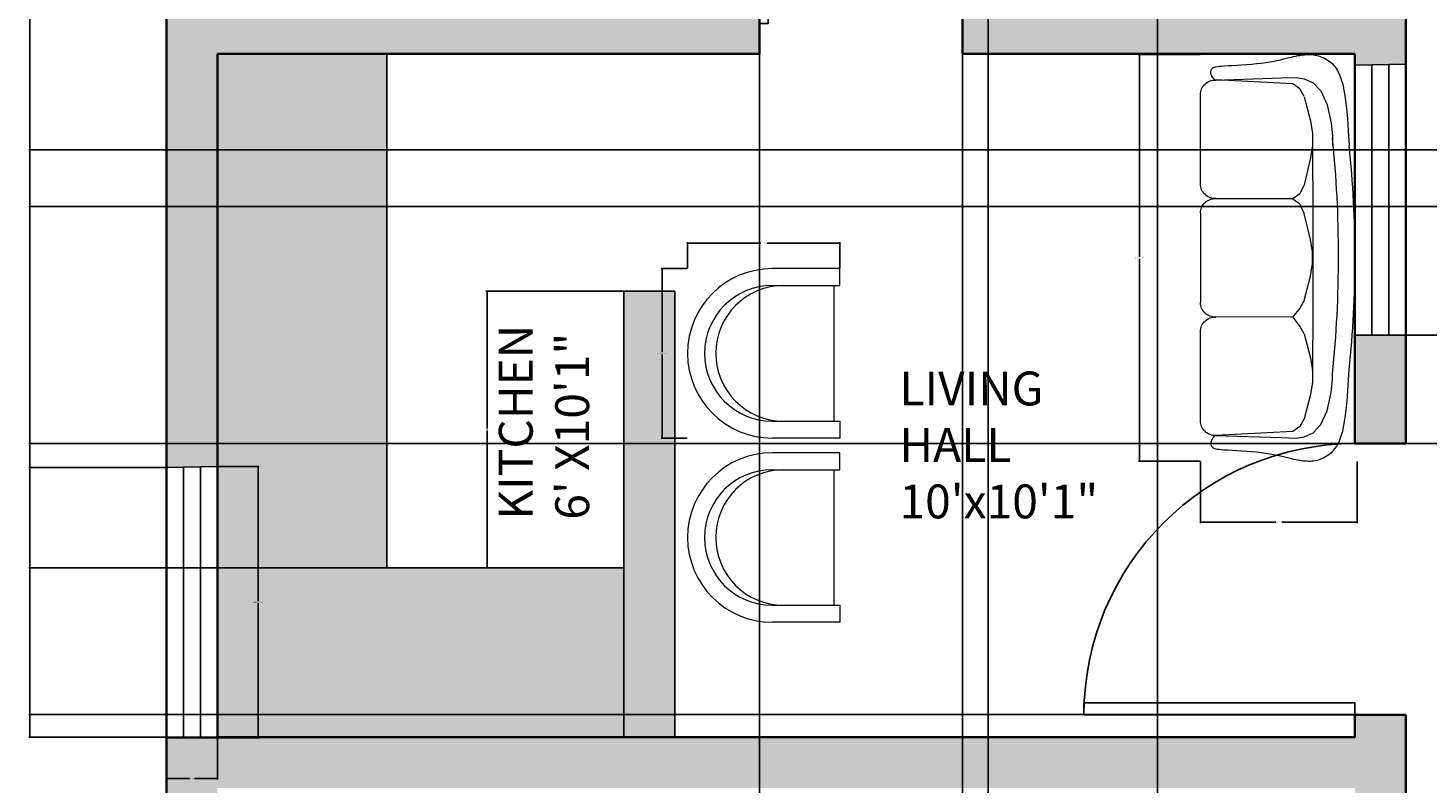
# Model space of a CAD drawing. Units: millimetres. Extents: x 2817 to 5038, y 1110 to 3565.
# Tile 10 of 21: x 2817 to 3065, y 1371 to 1505. Entities that reach past the tile are written whole.
import ezdxf

# ---------------------------------------------------------------- set-up
doc = ezdxf.new("R2010")
doc.units = ezdxf.units.MM
for name, color, linetype, lineweight in [('A-ANNO-DIMS', 2, 'Continuous', 18), ('A-AREA-IDEN', 7, 'Continuous', 18), ('A-FLOR-CASE', 7, 'Continuous', 25), ('A-WALL', 7, 'Continuous', 35), ('DOOR&WINDOW', 1, 'Continuous', 25), ('FURNITURE', 219, 'Continuous', 18)]:
    doc.layers.add(name, color=color, linetype=linetype, lineweight=lineweight)
doc.layers.add('A-FLOR-CASE-PATT', color=251, linetype='Continuous', lineweight=13, true_color=0x636466)
doc.layers.add('A-WALL-PATT', color=51, linetype='Continuous', lineweight=13, true_color=0xf7f281)
doc.styles.get("Standard").update_dxf_attribs({"font": 'arial.ttf'})
doc.dimstyles.get("Standard").update_dxf_attribs({"dimtxt": 0.18, "dimasz": 0.18, "dimexe": 0.18, "dimexo": 0.0625, "dimgap": 0.09, "dimtad": 0, "dimtih": 1, "dimtoh": 1, "dimdec": 4, "dimzin": 0, "dimdsep": 46, "dimtxsty": 'Standard', "dimcen": 0.09, "dimadec": 0, "dimazin": 0, "dimtfac": 1, "dimtdec": 4, "dimtofl": 0, "dimtmove": 0, "dimatfit": 3, "dimfxl": 1, "dimtolj": 1, "dimtzin": 0, "dimarcsym": 0})

# ---------------------------------------------------------------- blocks, each defined once
blk = doc.blocks.new('*U2')
for p, q in [((0, 0), (0, -6)), ((40, 0), (40, -6))]:
    blk.add_line(p, q)
blk.add_lwpolyline([(0, 0), (0, 40), (1.75, 40), (1.75, 0)], close=True)
blk.add_arc((0, 0), 40, 0, 90)
blk = doc.blocks.new('*U3')
for p, q in [((-40, 0), (-40, 6)), ((0, 0), (0, 6))]:
    blk.add_line(p, q)
blk.add_lwpolyline([(0, 0), (0, -40), (-1.75, -40), (-1.75, 0)], close=True)
blk.add_arc((0, 0), 40, 180, 270)
blk = doc.blocks.new('A$C2E47758B')
for p, q in [((168.6, 1918.7), (160.6, 1917.4)), ((176.5, 1919.5), (168.6, 1918.7)), ((184.4, 1919.9), (176.5, 1919.5)), ((192.3, 1919.9), (184.4, 1919.9)), ((200.2, 1919.6), (192.3, 1919.9)), ((208.2, 1919.1), (200.2, 1919.6)), ((216.4, 1918.3), (208.2, 1919.1)), ((224.7, 1917.3), (216.4, 1918.3)), ((61.4, 1854.6), (55.6, 1845.5)), ((67.4, 1862.7), (61.4, 1854.6)), ((73.8, 1870), (67.4, 1862.7)), ((80.6, 1876.8), (73.8, 1870)), ((87.8, 1883), (80.6, 1876.8)), ((95.4, 1888.9), (87.8, 1883)), ((103.3, 1894.2), (95.4, 1888.9)), ((111.3, 1899.1), (103.3, 1894.2)), ((119.6, 1903.5), (111.3, 1899.1)), ((127.9, 1907.3), (119.6, 1903.5)), ((136.2, 1910.7), (127.9, 1907.3)), ((144.4, 1913.5), (136.2, 1910.7)), ((152.6, 1915.7), (144.4, 1913.5)), ((160.6, 1917.4), (152.6, 1915.7)), ((233.3, 1916), (224.7, 1917.3)), ((242.3, 1914.5), (233.3, 1916)), ((251.8, 1912.6), (242.3, 1914.5)), ((261.8, 1910.5), (251.8, 1912.6)), ((272.6, 1908.1), (261.8, 1910.5)), ((284, 1905.3), (272.6, 1908.1)), ((296.4, 1902.3), (284, 1905.3)), ((309.7, 1899), (296.4, 1902.3)), ((324, 1895.5), (309.7, 1899)), ((339.5, 1892), (324, 1895.5)), ((356.2, 1888.6), (339.5, 1892)), ((374.2, 1885.2), (356.2, 1888.6)), ((393.6, 1882.1), (374.2, 1885.2)), ((414.5, 1879.2), (393.6, 1882.1)), ((436.8, 1876.8), (414.5, 1879.2)), ((460.2, 1874.7), (436.8, 1876.8)), ((484, 1872.9), (460.2, 1874.7)), ((507.6, 1871.3), (484, 1872.9)), ((530.4, 1869.9), (507.6, 1871.3)), ((551.8, 1868.7), (530.4, 1869.9)), ((571.3, 1867.6), (551.8, 1868.7)), ((588.2, 1866.5), (571.3, 1867.6)), ((602.2, 1865.5), (588.2, 1866.5)), ((613.4, 1864.4), (602.2, 1865.5)), ((622.2, 1863.3), (613.4, 1864.4)), ((628.9, 1862.1), (622.2, 1863.3)), ((634, 1860.9), (628.9, 1862.1)), ((637.8, 1859.6), (634, 1860.9)), ((640.6, 1858.2), (637.8, 1859.6)), ((642.9, 1856.7), (640.6, 1858.2)), ((644.9, 1855), (642.9, 1856.7)), ((646.7, 1853.2), (644.9, 1855)), ((648.3, 1851.2), (646.7, 1853.2)), ((35, 1796), (30.2, 1779.2)), ((39.9, 1810.7), (35, 1796)), ((44.9, 1823.7), (39.9, 1810.7)), ((50.2, 1835.3), (44.9, 1823.7)), ((55.6, 1845.5), (50.2, 1835.3)), ((169.1, 1786.1), (133.2, 1748)), ((211.4, 1805.2), (169.1, 1786.1)), ((249.5, 1811.5), (211.4, 1805.2)), ((319.3, 1809.4), (249.5, 1811.5)), ((266.4, 1781), (629.3, 1800.3)), ((633, 1799.3), (319.3, 1809.4)), ((626.2, 1798.6), (626.2, 1799)), ((627, 1799), (626.2, 1798.6)), ((633, 1799.3), (639.1, 1805.3)), ((639.1, 1805.3), (643.9, 1810.9)), ((643.9, 1810.9), (647.5, 1816.2)), ((647.5, 1816.2), (650, 1821.2)), ((649.7, 1849), (648.3, 1851.2)), ((650.8, 1846.6), (649.7, 1849)), ((650, 1821.2), (651.7, 1825.8)), ((651.7, 1843.9), (650.8, 1846.6)), ((652.4, 1840.9), (651.7, 1843.9)), ((651.7, 1825.8), (652.5, 1830.1)), ((652.8, 1837.6), (652.4, 1840.9)), ((652.5, 1830.1), (652.9, 1834)), ((652.9, 1834), (652.8, 1837.6)), ((21, 1734.4), (16.6, 1703.5)), ((25.6, 1759.2), (21, 1734.4)), ((30.2, 1779.2), (25.6, 1759.2)), ((133.2, 1748), (103.5, 1682.4)), ((211.4, 1721.7), (232.6, 1757.7)), ((232.6, 1757.7), (266.4, 1781)), ((232.6, 1757.7), (266.4, 1781)), ((12.3, 1665), (8.1, 1617.5)), ((16.6, 1703.5), (12.3, 1665)), ((103.5, 1682.4), (84.5, 1595.6)), ((8.1, 1617.5), (4, 1559.6)), ((84.5, 1595.6), (78.2, 1536.4)), ((4, 1559.6), (0, 1489.8)), ((78.2, 1536.4), (78.2, 1489.8)), ((78.2, 1515.4), (78.2, 1493.9)), ((211.4, 1169.1), (232.6, 1215)), ((181.8, 1046.7), (211.4, 1169.1)), ((702.1, 1170.7), (702.1, 749.2)), ((173.3, 987.5), (181.8, 1046.7)), ((173.3, 985.3), (173.3, 987.5)), ((173.3, 932.4), (173.3, 985.3)), ((181.8, 873.2), (173.3, 932.4)), ((211.4, 758.9), (181.8, 873.2)), ((211.4, 757.7), (232.6, 721.7)), ((232.6, 721.7), (266.4, 681.7)), ((232.6, 637.5), (266.4, 681.7)), ((266.4, 681.7), (629.3, 680.2)), ((266.4, 681.7), (629.3, 680.2)), ((627, 680.1), (626.2, 679.6)), ((626.2, 679.6), (626.2, 680)), ((627, 679.2), (626.2, 679.6)), ((626.2, 679.6), (626.2, 679.2)), ((211.4, 601.6), (181.8, 487.3)), ((211.4, 601.6), (232.6, 637.5)), ((702.1, 189.8), (702.1, 611.2)), ((181.8, 487.3), (173.3, 428)), ((4, 360.3), (0, 430.1)), ((78.2, 383.5), (78.2, 410.9)), ((173.3, 430.1), (173.3, 373)), ((173.3, 428), (173.3, 430.1)), ((8.1, 302.4), (4, 360.3)), ((84.5, 324.3), (78.2, 383.5)), ((173.3, 373), (181.8, 313.7)), ((12.3, 254.9), (8.1, 302.4)), ((103.5, 237.5), (84.5, 324.3)), ((181.8, 313.7), (211.4, 199.4)), ((16.6, 216.4), (12.3, 254.9)), ((21, 185.5), (16.6, 216.4)), ((133.2, 171.9), (103.5, 237.5)), ((211.4, 199.4), (232.6, 163.4)), ((25.6, 160.7), (21, 185.5)), ((30.2, 140.7), (25.6, 160.7)), ((35, 123.9), (30.2, 140.7)), ((169.1, 133.8), (133.2, 171.9)), ((211.4, 114.7), (169.1, 133.8)), ((232.6, 163.4), (266.4, 140.1)), ((266.4, 140.1), (629.3, 120.7)), ((39.9, 109.2), (35, 123.9)), ((44.9, 96.2), (39.9, 109.2)), ((50.2, 84.6), (44.9, 96.2)), ((55.6, 74.4), (50.2, 84.6)), ((61.4, 65.3), (55.6, 74.4)), ((249.5, 108.4), (211.4, 114.7)), ((319.3, 110.5), (249.5, 108.4)), ((633, 120.7), (319.3, 110.5)), ((626.2, 121.3), (626.2, 120.9)), ((627, 120.9), (626.2, 121.3)), ((633, 120.7), (639.1, 114.6)), ((639.1, 114.6), (643.9, 109)), ((643.9, 109), (647.5, 103.7)), ((646.7, 66.7), (644.9, 64.9)), ((648.3, 68.7), (646.7, 66.7)), ((647.5, 103.7), (650, 98.7)), ((649.7, 70.9), (648.3, 68.7)), ((650.8, 73.3), (649.7, 70.9)), ((650, 98.7), (651.7, 94.1)), ((651.7, 76), (650.8, 73.3)), ((651.7, 94.1), (652.5, 89.8)), ((652.4, 79), (651.7, 76)), ((652.8, 82.3), (652.4, 79)), ((652.5, 89.8), (652.9, 85.9)), ((652.9, 85.9), (652.8, 82.3)), ((67.4, 57.2), (61.4, 65.3)), ((73.8, 49.9), (67.4, 57.2)), ((80.6, 43.1), (73.8, 49.9)), ((87.8, 36.9), (80.6, 43.1)), ((95.4, 31.1), (87.8, 36.9)), ((103.3, 25.7), (95.4, 31.1)), ((111.3, 20.8), (103.3, 25.7)), ((119.6, 16.4), (111.3, 20.8)), ((127.9, 12.6), (119.6, 16.4)), ((136.2, 9.2), (127.9, 12.6)), ((144.4, 6.4), (136.2, 9.2)), ((152.6, 4.2), (144.4, 6.4)), ((160.6, 2.5), (152.6, 4.2)), ((168.6, 1.3), (160.6, 2.5)), ((176.5, 0.5), (168.6, 1.3)), ((184.4, 0), (176.5, 0.5)), ((192.3, 0), (184.4, 0)), ((200.2, 0.3), (192.3, 0)), ((208.2, 0.8), (200.2, 0.3)), ((216.4, 1.6), (208.2, 0.8)), ((224.7, 2.6), (216.4, 1.6)), ((233.3, 3.9), (224.7, 2.6)), ((242.3, 5.4), (233.3, 3.9)), ((251.8, 7.3), (242.3, 5.4)), ((261.8, 9.4), (251.8, 7.3)), ((272.6, 11.8), (261.8, 9.4)), ((284, 14.6), (272.6, 11.8)), ((296.4, 17.6), (284, 14.6)), ((309.7, 20.9), (296.4, 17.6)), ((324, 24.4), (309.7, 20.9)), ((339.5, 27.9), (324, 24.4)), ((356.2, 31.4), (339.5, 27.9)), ((374.2, 34.7), (356.2, 31.4)), ((393.6, 37.8), (374.2, 34.7)), ((414.5, 40.7), (393.6, 37.8)), ((436.8, 43.1), (414.5, 40.7)), ((460.2, 45.2), (436.8, 43.1)), ((484, 47), (460.2, 45.2)), ((507.6, 48.6), (484, 47)), ((530.4, 50), (507.6, 48.6)), ((551.8, 51.2), (530.4, 50)), ((571.3, 52.3), (551.8, 51.2)), ((588.2, 53.4), (571.3, 52.3)), ((602.2, 54.4), (588.2, 53.4)), ((613.4, 55.5), (602.2, 54.4)), ((622.2, 56.6), (613.4, 55.5)), ((628.9, 57.8), (622.2, 56.6)), ((634, 59), (628.9, 57.8)), ((637.8, 60.3), (634, 59)), ((640.6, 61.7), (637.8, 60.3)), ((642.9, 63.2), (640.6, 61.7)), ((644.9, 64.9), (642.9, 63.2))]:
    blk.add_line(p, q)
for points in [[(629.3, 1239.7), (266.4, 1238.2), (629.3, 1239.7, 0.429937), (702.1, 1308.7), (702.1, 1730.1, 0.429937), (629.3, 1799.2)], [(78.2, 410.9, -0.050936), (78.2, 1525.6, 12.167348)], [(0, 430.1, -0.05358), (0, 1489.8, 12.163767)], [(173.3, 1494, 0.004989), (173.3, 401.5, 0.847003)]]:
    blk.add_lwpolyline(points, format="xyb")
blk.add_lwpolyline([(211.4, 1720.5), (181.8, 1606.2), (173.3, 1546.9), (173.3, 1494), (173.3, 1491.9), (181.8, 1432.6), (211.4, 1304.3), (232.6, 1261.5), (266.4, 1238.2), (232.6, 1215)])
for centre, start, end in [((633, 1170.7), 0, 93.05866), ((633, 749.2), 266.94134, 360), ((633, 749.2), 266.94134, 360), ((633, 611.2), 0, 93.05866), ((633, 611.2), 0, 93.05866), ((633, 611.2), 0, 93.05866), ((633, 189.8), 266.94134, 360)]:
    blk.add_arc(centre, 69.1, start, end)
blk = doc.blocks.new('12PSTG07')
at = {"color": 0, "linetype": 'ByBlock'}
for p, q in [((0, 15), (-12, 15)), ((0, 12), (0, 15)), ((-12, 12), (0, 12)), ((-1, -12), (-1, 12)), ((-12, -12), (0, -12)), ((0, -12), (0, -15)), ((0, -15), (-12, -15))]:
    blk.add_line(p, q, dxfattribs=at)
for centre, radius in [((-12, 0), 15), ((-12, 0), 12), ((-10, 0), 12)]:
    blk.add_arc(centre, radius, 90, 270, dxfattribs=at)
blk = doc.blocks.new('WIN-4FT')
for p, q in [((0, 47.85), (9, 48)), ((0, 0), (0, 47.85)), ((3, 0), (3, 47.85)), ((6, 48), (6, 0)), ((9, 48), (9, 0)), ((9, 0), (0, 0))]:
    blk.add_line(p, q)
blk = doc.blocks.new('*D14')
at = {"layer": 'A-ANNO-DIMS', "color": 0, "lineweight": -2, "transparency": 16777216}
for p, q in [((2850.8, 1427.36), (2858.12, 1427.36)), ((2857.94, 1427.18), (2857.94, 1403.55)), ((2857.94, 1379.54), (2857.94, 1403.18)), ((2850.8, 1379.36), (2858.12, 1379.36))]:
    blk.add_line(p, q, dxfattribs=at)
for points in [[(2857.91, 1427.18), (2857.97, 1427.18), (2857.94, 1427.36)], [(2857.91, 1379.54), (2857.97, 1379.54), (2857.94, 1379.36)]]:
    blk.add_solid(points, dxfattribs=at)
at = {"layer": 'Defpoints', "color": 0, "lineweight": -2, "transparency": 16777216}
for p in [(2850.74, 1427.36), (2857.94, 1427.36), (2850.74, 1379.36)]:
    blk.add_point(p, dxfattribs=at)
at = {"layer": 'A-ANNO-DIMS', "color": 0, "transparency": 16777216, "insert": (2857.94, 1403.36), "char_height": 0.18, "attachment_point": 5}
blk.add_mtext('\\A1;WINDOW 48 TYP.', dxfattribs=at)
blk = doc.blocks.new('*D15')
at = {"layer": 'A-ANNO-DIMS', "color": 0, "lineweight": -2, "transparency": 16777216}
for p, q in [((2841.74, 1379.3), (2841.74, 1371.98)), ((2850.74, 1379.3), (2850.74, 1371.98)), ((2841.92, 1372.16), (2845.78, 1372.16)), ((2850.56, 1372.16), (2846.7, 1372.16))]:
    blk.add_line(p, q, dxfattribs=at)
for points in [[(2841.92, 1372.19), (2841.92, 1372.13), (2841.74, 1372.16)], [(2850.56, 1372.19), (2850.56, 1372.13), (2850.74, 1372.16)]]:
    blk.add_solid(points, dxfattribs=at)
at = {"layer": 'Defpoints', "color": 0, "lineweight": -2, "transparency": 16777216}
for p in [(2841.74, 1379.36), (2850.74, 1379.36), (2850.74, 1372.16)]:
    blk.add_point(p, dxfattribs=at)
at = {"layer": 'A-ANNO-DIMS', "color": 0, "transparency": 16777216, "insert": (2846.24, 1372.16), "char_height": 0.18, "attachment_point": 5}
blk.add_mtext('\\A1;9 TYP.', dxfattribs=at)
blk = doc.blocks.new('*D20')
at = {"layer": 'A-ANNO-DIMS', "color": 0, "lineweight": -2, "transparency": 16777216}
for p, q in [((3024.81, 1500.32), (3013.9, 1500.32)), ((3014.08, 1500.14), (3014.08, 1464.52)), ((3014.08, 1428.52), (3014.08, 1464.15)), ((3024.81, 1428.34), (3013.9, 1428.34))]:
    blk.add_line(p, q, dxfattribs=at)
for points in [[(3014.05, 1500.14), (3014.11, 1500.14), (3014.08, 1500.32)], [(3014.05, 1428.52), (3014.11, 1428.52), (3014.08, 1428.34)]]:
    blk.add_solid(points, dxfattribs=at)
at = {"layer": 'Defpoints', "color": 0, "lineweight": -2, "transparency": 16777216}
for p in [(3014.08, 1500.32), (3024.87, 1500.32), (3024.87, 1428.34)]:
    blk.add_point(p, dxfattribs=at)
at = {"layer": 'A-ANNO-DIMS', "color": 0, "transparency": 16777216, "insert": (3014.08, 1464.33), "char_height": 0.18, "attachment_point": 5}
blk.add_mtext('\\A1;SOFA 72 TYP.', dxfattribs=at)
blk = doc.blocks.new('*D21')
at = {"layer": 'A-ANNO-DIMS', "color": 0, "lineweight": -2, "transparency": 16777216}
for p, q in [((3024.87, 1428.28), (3024.87, 1417.37)), ((3052.62, 1428.28), (3052.62, 1417.37)), ((3025.05, 1417.55), (3038.21, 1417.55)), ((3052.44, 1417.55), (3039.27, 1417.55))]:
    blk.add_line(p, q, dxfattribs=at)
for points in [[(3025.05, 1417.58), (3025.05, 1417.52), (3024.87, 1417.55)], [(3052.44, 1417.58), (3052.44, 1417.52), (3052.62, 1417.55)]]:
    blk.add_solid(points, dxfattribs=at)
at = {"layer": 'Defpoints', "color": 0, "lineweight": -2, "transparency": 16777216}
for p in [(3024.87, 1428.34), (3052.62, 1428.34), (3024.87, 1417.55)]:
    blk.add_point(p, dxfattribs=at)
at = {"layer": 'A-ANNO-DIMS', "color": 0, "transparency": 16777216, "insert": (3038.74, 1417.55), "char_height": 0.18, "attachment_point": 5}
blk.add_mtext('\\A1;28 TYP.', dxfattribs=at)
blk = doc.blocks.new('*D22')
at = {"layer": 'A-ANNO-DIMS', "color": 0, "lineweight": -2, "transparency": 16777216}
for p, q in [((2933.95, 1462.41), (2929.34, 1462.41)), ((2929.52, 1462.23), (2929.52, 1447.6)), ((2929.52, 1432.59), (2929.52, 1447.23)), ((2933.95, 1432.41), (2929.34, 1432.41))]:
    blk.add_line(p, q, dxfattribs=at)
for points in [[(2929.49, 1462.23), (2929.55, 1462.23), (2929.52, 1462.41)], [(2929.49, 1432.59), (2929.55, 1432.59), (2929.52, 1432.41)]]:
    blk.add_solid(points, dxfattribs=at)
at = {"layer": 'Defpoints', "color": 0, "lineweight": -2, "transparency": 16777216}
for p in [(2929.52, 1462.41), (2934.02, 1462.41), (2934.02, 1432.41)]:
    blk.add_point(p, dxfattribs=at)
at = {"layer": 'A-ANNO-DIMS', "color": 0, "transparency": 16777216, "insert": (2929.52, 1447.41), "char_height": 0.18, "attachment_point": 5}
blk.add_mtext('\\A1;CHAIR 30 TYP.', dxfattribs=at)
blk = doc.blocks.new('*D23')
at = {"layer": 'A-ANNO-DIMS', "color": 0, "lineweight": -2, "transparency": 16777216}
for p, q in [((2934.02, 1462.47), (2934.02, 1467.09)), ((2934.2, 1466.91), (2946.99, 1466.91)), ((2960.84, 1466.91), (2948.05, 1466.91)), ((2961.02, 1462.47), (2961.02, 1467.09))]:
    blk.add_line(p, q, dxfattribs=at)
for points in [[(2934.2, 1466.94), (2934.2, 1466.88), (2934.02, 1466.91)], [(2960.84, 1466.94), (2960.84, 1466.88), (2961.02, 1466.91)]]:
    blk.add_solid(points, dxfattribs=at)
at = {"layer": 'Defpoints', "color": 0, "lineweight": -2, "transparency": 16777216}
for p in [(2961.02, 1466.91), (2934.02, 1462.41), (2961.02, 1462.41)]:
    blk.add_point(p, dxfattribs=at)
at = {"layer": 'A-ANNO-DIMS', "color": 0, "transparency": 16777216, "insert": (2947.52, 1466.91), "char_height": 0.18, "attachment_point": 5}
blk.add_mtext('\\A1;27 TYP.', dxfattribs=at)
blk = doc.blocks.new('*D33')
at = {"layer": 'A-ANNO-DIMS', "color": 0, "lineweight": -2, "transparency": 16777216}
for p, q in [((2841.68, 1520.76), (2817.31, 1520.76)), ((2817.49, 1520.58), (2817.49, 1474.17)), ((2817.49, 1427.4), (2817.49, 1473.81)), ((2841.68, 1427.22), (2817.31, 1427.22))]:
    blk.add_line(p, q, dxfattribs=at)
for points in [[(2817.46, 1520.58), (2817.52, 1520.58), (2817.49, 1520.76)], [(2817.46, 1427.4), (2817.52, 1427.4), (2817.49, 1427.22)]]:
    blk.add_solid(points, dxfattribs=at)
at = {"layer": 'Defpoints', "color": 0, "lineweight": -2, "transparency": 16777216}
for p in [(2817.49, 1520.76), (2841.74, 1520.76), (2841.74, 1427.22)]:
    blk.add_point(p, dxfattribs=at)
at = {"layer": 'A-ANNO-DIMS', "color": 0, "transparency": 16777216, "insert": (2817.49, 1473.99), "char_height": 0.18, "attachment_point": 5}
blk.add_mtext('\\A1;93.54', dxfattribs=at)
blk = doc.blocks.new('*D34')
at = {"layer": 'A-ANNO-DIMS', "color": 0, "lineweight": -2, "transparency": 16777216}
for p, q in [((2946.74, 1500.37), (2946.74, 1110.01)), ((2982.74, 1500.37), (2982.74, 1110.01)), ((2946.92, 1110.19), (2964.52, 1110.19)), ((2982.56, 1110.19), (2964.96, 1110.19))]:
    blk.add_line(p, q, dxfattribs=at)
for points in [[(2946.92, 1110.22), (2946.92, 1110.16), (2946.74, 1110.19)], [(2982.56, 1110.22), (2982.56, 1110.16), (2982.74, 1110.19)]]:
    blk.add_solid(points, dxfattribs=at)
at = {"layer": 'Defpoints', "color": 0, "lineweight": -2, "transparency": 16777216}
for p in [(2946.74, 1500.44), (2982.74, 1500.44), (2982.74, 1110.19)]:
    blk.add_point(p, dxfattribs=at)
at = {"layer": 'A-ANNO-DIMS', "color": 0, "transparency": 16777216, "insert": (2964.74, 1110.19), "char_height": 0.18, "attachment_point": 5}
blk.add_mtext('\\A1;36', dxfattribs=at)
blk = doc.blocks.new('*D35')
at = {"layer": 'A-ANNO-DIMS', "color": 0, "lineweight": -2, "transparency": 16777216}
for p, q in [((2987.24, 1605.37), (2987.24, 1110.01)), ((3017.24, 1605.37), (3017.24, 1110.01)), ((2987.42, 1110.19), (3002.02, 1110.19)), ((3017.06, 1110.19), (3002.46, 1110.19))]:
    blk.add_line(p, q, dxfattribs=at)
for points in [[(2987.42, 1110.22), (2987.42, 1110.16), (2987.24, 1110.19)], [(3017.06, 1110.22), (3017.06, 1110.16), (3017.24, 1110.19)]]:
    blk.add_solid(points, dxfattribs=at)
at = {"layer": 'Defpoints', "color": 0, "lineweight": -2, "transparency": 16777216}
for p in [(2987.24, 1605.44), (3017.24, 1605.44), (3017.24, 1110.19)]:
    blk.add_point(p, dxfattribs=at)
at = {"layer": 'A-ANNO-DIMS', "color": 0, "transparency": 16777216, "insert": (3002.24, 1110.19), "char_height": 0.18, "attachment_point": 5}
blk.add_mtext('\\A1;30', dxfattribs=at)
blk = doc.blocks.new('*D36')
at = {"layer": 'A-ANNO-DIMS', "color": 0, "lineweight": -2, "transparency": 16777216}
for p, q in [((3052.18, 1431.44), (2817.31, 1431.44)), ((2817.49, 1431.26), (2817.49, 1407.62)), ((2817.49, 1383.62), (2817.49, 1407.25)), ((3052.18, 1383.44), (2817.31, 1383.44))]:
    blk.add_line(p, q, dxfattribs=at)
for points in [[(2817.46, 1431.26), (2817.52, 1431.26), (2817.49, 1431.44)], [(2817.46, 1383.62), (2817.52, 1383.62), (2817.49, 1383.44)]]:
    blk.add_solid(points, dxfattribs=at)
at = {"layer": 'Defpoints', "color": 0, "lineweight": -2, "transparency": 16777216}
for p in [(2817.49, 1431.44), (3052.24, 1431.44), (3052.24, 1383.44)]:
    blk.add_point(p, dxfattribs=at)
at = {"layer": 'A-ANNO-DIMS', "color": 0, "transparency": 16777216, "insert": (2817.49, 1407.44), "char_height": 0.18, "attachment_point": 5}
blk.add_mtext('\\A1;48', dxfattribs=at)
blk = doc.blocks.new('*D38')
at = {"layer": 'A-ANNO-DIMS', "color": 0, "lineweight": -2, "transparency": 16777216}
for p, q in [((3110.18, 1573.44), (2817.31, 1573.44)), ((2817.49, 1573.26), (2817.49, 1523.62)), ((2817.49, 1473.62), (2817.49, 1523.25)), ((3105.68, 1473.44), (2817.31, 1473.44))]:
    blk.add_line(p, q, dxfattribs=at)
for points in [[(2817.46, 1573.26), (2817.52, 1573.26), (2817.49, 1573.44)], [(2817.46, 1473.62), (2817.52, 1473.62), (2817.49, 1473.44)]]:
    blk.add_solid(points, dxfattribs=at)
at = {"layer": 'Defpoints', "color": 0, "lineweight": -2, "transparency": 16777216}
for p in [(2817.49, 1573.44), (3110.24, 1573.44), (3105.74, 1473.44)]:
    blk.add_point(p, dxfattribs=at)
at = {"layer": 'A-ANNO-DIMS', "color": 0, "transparency": 16777216, "insert": (2817.49, 1523.44), "char_height": 0.18, "attachment_point": 5}
blk.add_mtext('\\A1;100', dxfattribs=at)
blk = doc.blocks.new('*D40')
at = {"layer": 'A-ANNO-DIMS', "color": 0, "lineweight": -2, "transparency": 16777216}
for p, q in [((3182.18, 1483.44), (2817.31, 1483.44)), ((2817.49, 1483.26), (2817.49, 1478.62)), ((2817.49, 1473.62), (2817.49, 1478.25)), ((3182.18, 1473.44), (2817.31, 1473.44))]:
    blk.add_line(p, q, dxfattribs=at)
for points in [[(2817.46, 1483.26), (2817.52, 1483.26), (2817.49, 1483.44)], [(2817.46, 1473.62), (2817.52, 1473.62), (2817.49, 1473.44)]]:
    blk.add_solid(points, dxfattribs=at)
at = {"layer": 'Defpoints', "color": 0, "lineweight": -2, "transparency": 16777216}
for p in [(2817.49, 1483.44), (3182.24, 1483.44), (3182.24, 1473.44)]:
    blk.add_point(p, dxfattribs=at)
at = {"layer": 'A-ANNO-DIMS', "color": 0, "transparency": 16777216, "insert": (2817.49, 1478.44), "char_height": 0.18, "attachment_point": 5}
blk.add_mtext('\\A1;10', dxfattribs=at)
blk = doc.blocks.new('*D43')
at = {"layer": 'A-ANNO-DIMS', "color": 0, "lineweight": -2, "transparency": 16777216}
for p, q in [((2922.68, 1409.44), (2817.31, 1409.44)), ((2817.49, 1409.26), (2817.49, 1394.62)), ((2817.49, 1379.62), (2817.49, 1394.25)), ((2922.68, 1379.44), (2817.31, 1379.44))]:
    blk.add_line(p, q, dxfattribs=at)
for points in [[(2817.46, 1409.26), (2817.52, 1409.26), (2817.49, 1409.44)], [(2817.46, 1379.62), (2817.52, 1379.62), (2817.49, 1379.44)]]:
    blk.add_solid(points, dxfattribs=at)
at = {"layer": 'Defpoints', "color": 0, "lineweight": -2, "transparency": 16777216}
for p in [(2922.74, 1409.44), (2817.49, 1379.44), (2922.74, 1379.44)]:
    blk.add_point(p, dxfattribs=at)
at = {"layer": 'A-ANNO-DIMS', "color": 0, "transparency": 16777216, "insert": (2817.49, 1394.44), "char_height": 0.18, "attachment_point": 5}
blk.add_mtext('\\A1;30', dxfattribs=at)
blk = doc.blocks.new('*D44')
at = {"layer": 'A-ANNO-DIMS', "color": 0, "lineweight": -2, "transparency": 16777216}
for p, q in [((2922.68, 1458.44), (2898.31, 1458.44)), ((2898.49, 1458.26), (2898.49, 1434.12)), ((2898.49, 1409.62), (2898.49, 1433.75)), ((2922.68, 1409.44), (2898.31, 1409.44))]:
    blk.add_line(p, q, dxfattribs=at)
for points in [[(2898.46, 1458.26), (2898.52, 1458.26), (2898.49, 1458.44)], [(2898.46, 1409.62), (2898.52, 1409.62), (2898.49, 1409.44)]]:
    blk.add_solid(points, dxfattribs=at)
at = {"layer": 'Defpoints', "color": 0, "lineweight": -2, "transparency": 16777216}
for p in [(2898.49, 1458.44), (2922.74, 1458.44), (2922.74, 1409.44)]:
    blk.add_point(p, dxfattribs=at)
at = {"layer": 'A-ANNO-DIMS', "color": 0, "transparency": 16777216, "insert": (2898.49, 1433.94), "char_height": 0.18, "attachment_point": 5}
blk.add_mtext('\\A1;49', dxfattribs=at)
blk = doc.blocks.new('*D49')
at = {"layer": 'A-ANNO-DIMS', "color": 0, "lineweight": -2, "transparency": 16777216}
for p, q in [((3061.3, 1450.61), (3085.67, 1450.61)), ((3085.49, 1450.43), (3085.49, 1441.21)), ((3085.49, 1431.62), (3085.49, 1440.84)), ((3061.3, 1431.44), (3085.67, 1431.44))]:
    blk.add_line(p, q, dxfattribs=at)
for points in [[(3085.46, 1450.43), (3085.52, 1450.43), (3085.49, 1450.61)], [(3085.46, 1431.62), (3085.52, 1431.62), (3085.49, 1431.44)]]:
    blk.add_solid(points, dxfattribs=at)
at = {"layer": 'Defpoints', "color": 0, "lineweight": -2, "transparency": 16777216}
for p in [(3061.24, 1450.61), (3061.24, 1431.44), (3085.49, 1431.44)]:
    blk.add_point(p, dxfattribs=at)
at = {"layer": 'A-ANNO-DIMS', "color": 0, "transparency": 16777216, "insert": (3085.49, 1441.02), "char_height": 0.18, "attachment_point": 5}
blk.add_mtext('\\A1;19.177', dxfattribs=at)

msp = doc.modelspace()

# ---------------------------------------------------------------- hatches: boundary and pattern name
at = {"layer": 'A-FLOR-CASE-PATT'}
h = msp.add_hatch(color=256, dxfattribs=at)
h.dxf.hatch_style = 1
h.paths.add_polyline_path([(2850.7393, 1379.4357), (2922.7393, 1379.4357), (2922.7393, 1409.4357), (2880.7393, 1409.4357), (2880.7393, 1500.4357), (2850.7393, 1500.4357)])
h = msp.add_hatch(color=256, dxfattribs=at)
h.dxf.hatch_style = 1
h.paths.add_polyline_path([(2931.7393, 1458.4357), (2922.7393, 1458.4357), (2922.7393, 1379.4357), (2931.7393, 1379.4357)])
h.paths.add_polyline_path([(2931.7393, 1211.4357), (2922.7393, 1211.4357), (2922.7393, 1143.4357), (2931.7393, 1143.4357)])
h = msp.add_hatch(color=256, dxfattribs=at)
h.dxf.hatch_style = 1
h.paths.add_polyline_path([(2931.7393, 1458.4357), (2922.7393, 1458.4357), (2922.7393, 1379.4357), (2931.7393, 1379.4357)])
h.paths.add_polyline_path([(2931.7393, 1211.4357), (2922.7393, 1211.4357), (2922.7393, 1143.4357), (2931.7393, 1143.4357)])
at = {"layer": 'A-WALL-PATT'}
h = msp.add_hatch(color=256, dxfattribs=at)
h.dxf.hatch_style = 1
h.paths.add_polyline_path([(3186.7393, 1614.4357), (2841.7393, 1614.4357), (2841.7393, 1568.614), (2850.7393, 1568.7609), (2850.7393, 1605.4357), (2982.7393, 1605.4357), (2991.7393, 1605.4357), (3052.2393, 1605.4357), (3052.2393, 1573.7835), (3061.2393, 1573.7835), (3061.2393, 1605.4357), (3182.2393, 1605.4357), (3182.2393, 1143.4357), (3181.2393, 1143.4357), (3181.2393, 1134.4357), (3186.7393, 1134.4357)])
h.paths.add_polyline_path([(3061.2393, 1143.4357), (3061.2393, 1147.4357), (3052.2393, 1147.4357), (3052.2393, 1143.4357), (2850.7393, 1143.4357), (2850.7393, 1145.2996), (2841.7393, 1145.2996), (2841.7393, 1134.4357), (3061.2393, 1134.4357)], flags=17)
h.paths.add_polyline_path([(2850.7393, 1265.4357), (2946.7393, 1265.4357), (2946.7393, 1270.8357), (2946.7393, 1274.4357), (2850.7393, 1274.4357), (2850.7381, 1274.4357), (2850.7381, 1274.2564), (2841.7393, 1274.2564), (2841.7393, 1193.1527), (2850.7393, 1193.2996)], flags=17)
h.paths.add_polyline_path([(3061.2393, 1299.098), (3052.2393, 1299.098), (3052.2393, 1274.4357), (2991.7393, 1274.4357), (2991.7393, 1340.4357), (2982.7393, 1340.4357), (2982.7393, 1274.4357), (2982.7393, 1265.4357), (3052.2393, 1265.4357), (3052.2393, 1259.143), (3061.2393, 1259.2899)], flags=17)
h.paths.add_polyline_path([(3061.2393, 1383.4357), (3052.2393, 1383.4357), (3052.2393, 1379.4357), (2931.7393, 1379.4357), (2922.7393, 1379.4357), (2850.7393, 1379.4357), (2850.7381, 1379.4357), (2850.7381, 1379.3646), (2841.7393, 1379.3646), (2841.7393, 1322.1095), (2850.7393, 1322.2564), (2850.7393, 1370.4357), (2982.7393, 1370.4357), (2987.2393, 1370.4357), (3017.2393, 1370.4357), (3052.2393, 1370.4357), (3052.2393, 1323.098), (3061.2393, 1323.098)], flags=17)
h = msp.add_hatch(color=256, dxfattribs=at)
h.dxf.hatch_style = 1
h.paths.add_polyline_path([(3061.2393, 1549.7835), (3052.2393, 1549.7835), (3052.2393, 1509.4357), (2991.7393, 1509.4357), (2991.7393, 1575.4357), (2982.7393, 1575.4357), (2982.7393, 1509.4357), (2982.7393, 1500.4357), (3052.2393, 1500.4357), (3052.2393, 1498.4661), (3061.2393, 1498.613)])
h.paths.add_polyline_path([(2946.7393, 1505.8357), (2946.7393, 1509.4357), (2850.7393, 1509.4357), (2850.7393, 1520.7609), (2841.7393, 1520.7609), (2841.7393, 1427.2177), (2850.7393, 1427.3646), (2850.7393, 1500.4357), (2922.7393, 1500.4357), (2931.7393, 1500.4357), (2946.7393, 1500.4357)])
h.paths.add_polyline_path([(3061.2393, 1450.613), (3052.2393, 1450.613), (3052.2393, 1431.4357), (3059.4393, 1431.4357), (3061.2393, 1431.4357)])
h.paths.add_polyline_path([(3061.2393, 1211.2899), (3052.2393, 1211.2899), (3052.2393, 1195.4357), (3059.4393, 1195.4357), (3061.2393, 1195.4357)])

# ---------------------------------------------------------------- linework, layer by layer
at = {"layer": 'A-FLOR-CASE'}
for p, q in [((2880.7393, 1409.4357), (2880.7393, 1500.4357)), ((2922.7393, 1379.4357), (2922.7393, 1458.4357)), ((2922.7393, 1458.4357), (2931.7393, 1458.4357)), ((2931.7393, 1379.4357), (2931.7393, 1458.4357)), ((2880.7393, 1409.4357), (2922.7393, 1409.4357))]:
    msp.add_line(p, q, dxfattribs=at)
at = {"layer": 'A-WALL'}
for p, q in [((2841.7393, 1134.4357), (2841.7393, 1614.4357)), ((3061.2393, 1605.4357), (3061.2393, 1431.4357)), ((2946.7393, 1500.4357), (2946.7393, 1509.4357)), ((2982.7393, 1500.4357), (2982.7393, 1509.4357)), ((2850.7393, 1500.4357), (2922.7393, 1500.4357)), ((2850.7393, 1379.4357), (2850.7393, 1500.4357)), ((2922.7393, 1500.4357), (2931.7393, 1500.4357)), ((2931.7393, 1500.4357), (2946.7393, 1500.4357)), ((2982.7393, 1500.4357), (3052.2393, 1500.4357)), ((3052.2393, 1500.4357), (3052.2393, 1431.4357)), ((3052.2393, 1431.4357), (3061.2393, 1431.4357)), ((3052.2393, 1383.4357), (3061.2393, 1383.4357)), ((3052.2393, 1383.4357), (3052.2393, 1379.4357)), ((3061.2393, 1383.4357), (3061.2393, 1195.4357)), ((2850.7393, 1379.4357), (2922.7393, 1379.4357)), ((2922.7393, 1379.4357), (2931.7393, 1379.4357)), ((2931.7393, 1379.4357), (3052.2393, 1379.4357))]:
    msp.add_line(p, q, dxfattribs=at)

# ---------------------------------------------------------------- block references
at = {"layer": 'DOOR&WINDOW', "xscale": 0.9, "yscale": 0.9, "zscale": 0.9}
msp.add_blockref('*U2', (2946.7393, 1505.8357), dxfattribs=at)
at = {"layer": 'DOOR&WINDOW'}
for p in [(3052.2393, 1450.613), (2841.7381, 1379.3645)]:
    msp.add_blockref('WIN-4FT', p, dxfattribs=at)
at = {"layer": 'DOOR&WINDOW', "xscale": 1.199999999999999, "yscale": 1.199999999999999, "zscale": 1.199999999999999, "rotation": 270}
msp.add_blockref('*U3', (3052.2393, 1383.4357), dxfattribs=at)
at = {"layer": 'FURNITURE', "xscale": -0.0374923371980192, "yscale": 0.0374923371980192, "zscale": 0.0374923371980192}
msp.add_blockref('A$C2E47758B', (3051.1964, 1428.3424), dxfattribs=at)
at = {"layer": 'FURNITURE'}
for p in [(2961.016, 1447.4119), (2961.016, 1414.8126)]:
    msp.add_blockref('12PSTG07', p, dxfattribs=at)

# ---------------------------------------------------------------- texts
at = {"layer": 'A-AREA-IDEN', "insert": (2900.5784, 1417.953), "char_height": 6, "attachment_point": 1, "rotation": 90}
msp.add_mtext_dynamic_manual_height_columns('KITCHEN\\P6\' X10\'1"', width=42.068425, gutter_width=12.5, heights=[0], dxfattribs=at)
at = {"layer": 'A-AREA-IDEN', "insert": (2971.5514, 1444.1958), "char_height": 6, "attachment_point": 1}
msp.add_mtext_dynamic_manual_height_columns('LIVING HALL\\P10\'x10\'1"', width=42.068425, gutter_width=12.5, heights=[0], dxfattribs=at)

# ---------------------------------------------------------------- dimensions: what is measured, and where the dimension line sits
at = {"layer": 'A-ANNO-DIMS'}
for base, p1, p2, picture, middle in [((3017.2393, 1110.1857), (2987.2393, 1605.4357), (3017.2393, 1605.4357), '*D35', (3002.2393, 1110.1857)), ((2982.7393, 1110.1857), (2946.7393, 1500.4357), (2982.7393, 1500.4357), '*D34', (2964.7393, 1110.1857))]:
    dim = msp.add_linear_dim(base=base, p1=p1, p2=p2, dimstyle='Standard', override={"dimdec": 0, "dimlfac": 1, "dimrnd": 0, "dimzin": 0, "dimdsep": 46, "dimlunit": 2}, dxfattribs=at)
    dim.commit()
    dim.dimension.update_dxf_attribs({"geometry": picture, "text_midpoint": middle})
for base, p1, p2, angle, override, picture, middle in [((2817.4881, 1573.4357), (3105.7393, 1473.4357), (3110.2393, 1573.4357), 90, {"dimdec": 0, "dimlfac": 1, "dimrnd": 0, "dimzin": 0, "dimdsep": 46, "dimlunit": 2}, '*D38', (2817.4881, 1523.4357)), ((2817.4881, 1520.7609), (2841.7393, 1427.2177), (2841.7381, 1520.7609), 90, {"dimdec": 2, "dimlfac": 1, "dimrnd": 0, "dimzin": 0, "dimdsep": 46, "dimlunit": 2}, '*D33', (2817.4881, 1473.9893)), ((2817.4881, 1483.4357), (3182.2393, 1473.4357), (3182.2393, 1483.4357), 90, {"dimdec": 0, "dimlfac": 1, "dimrnd": 0, "dimzin": 0, "dimdsep": 46, "dimlunit": 2}, '*D40', (2817.4881, 1478.4357)), ((2898.4893, 1458.4357), (2922.7393, 1409.4357), (2922.7393, 1458.4357), 90, {"dimdec": 0, "dimlfac": 1, "dimrnd": 0, "dimzin": 0, "dimdsep": 46, "dimlunit": 2}, '*D44', (2898.4893, 1433.9357)), ((3085.4893, 1431.4357), (3061.2393, 1450.613), (3061.2393, 1431.4357), 270, {"dimdec": 3, "dimlfac": 1, "dimrnd": 0, "dimzin": 0, "dimdsep": 46, "dimlunit": 2}, '*D49', (3085.4893, 1441.0244)), ((2817.4881, 1431.4357), (3052.2393, 1383.4357), (3052.2393, 1431.4357), 90, {"dimdec": 0, "dimlfac": 1, "dimrnd": 0, "dimzin": 0, "dimdsep": 46, "dimlunit": 2}, '*D36', (2817.4881, 1407.4357)), ((2817.4881, 1379.4357), (2922.7393, 1409.4357), (2922.7393, 1379.4357), 90, {"dimdec": 0, "dimlfac": 1, "dimrnd": 0, "dimzin": 0, "dimdsep": 46, "dimlunit": 2}, '*D43', (2817.4881, 1394.4357))]:
    dim = msp.add_linear_dim(base=base, p1=p1, p2=p2, angle=angle, dimstyle='Standard', override=override, dxfattribs=at)
    dim.commit()
    dim.dimension.update_dxf_attribs({"geometry": picture, "text_midpoint": middle})
for base, p1, p2, angle, text, picture, middle in [((3014.0755, 1500.324), (3024.8728, 1428.3424), (3024.8728, 1500.324), 90, 'SOFA <> TYP.', '*D20', (3014.0755, 1464.3332)), ((2929.516, 1462.4119), (2934.016, 1432.4119), (2934.016, 1462.4119), 90, 'CHAIR <> TYP.', '*D22', (2929.516, 1447.4119)), ((2857.9381, 1427.3646), (2850.7381, 1379.3645), (2850.7381, 1427.3646), 90, 'WINDOW <> TYP.', '*D14', (2857.9381, 1403.3645)), ((3024.8728, 1417.5451), (3052.6156, 1428.3424), (3024.8728, 1428.3424), 180, '<> TYP.', '*D21', (3038.7442, 1417.5451))]:
    dim = msp.add_linear_dim(base=base, p1=p1, p2=p2, angle=angle, text=text, dimstyle='Standard', override={"dimdec": 0, "dimlfac": 1, "dimrnd": 0, "dimzin": 0, "dimdsep": 46, "dimlunit": 2}, dxfattribs=at)
    dim.commit()
    dim.dimension.update_dxf_attribs({"geometry": picture, "text_midpoint": middle})
for base, p1, p2, picture, middle in [((2961.016, 1466.9119), (2934.016, 1462.4119), (2961.016, 1462.4119), '*D23', (2947.516, 1466.9119)), ((2850.7381, 1372.1645), (2841.7381, 1379.3645), (2850.7381, 1379.3645), '*D15', (2846.2381, 1372.1645))]:
    dim = msp.add_linear_dim(base=base, p1=p1, p2=p2, text='<> TYP.', dimstyle='Standard', override={"dimdec": 0, "dimlfac": 1, "dimrnd": 0, "dimzin": 0, "dimdsep": 46, "dimlunit": 2}, dxfattribs=at)
    dim.commit()
    dim.dimension.update_dxf_attribs({"geometry": picture, "text_midpoint": middle})

doc.saveas('drawing.dxf')
